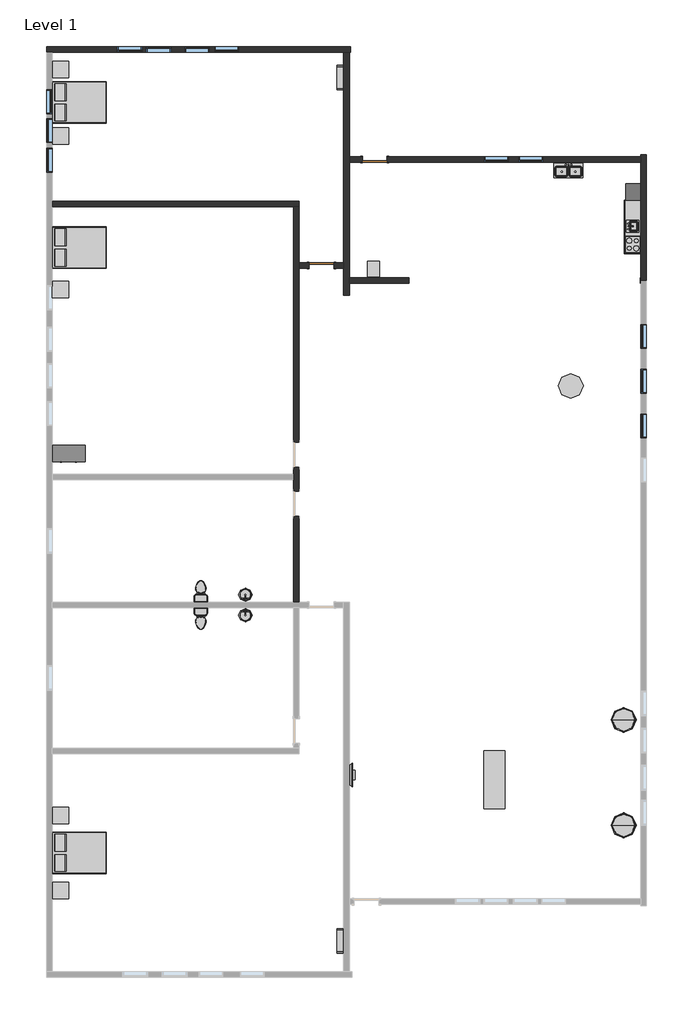
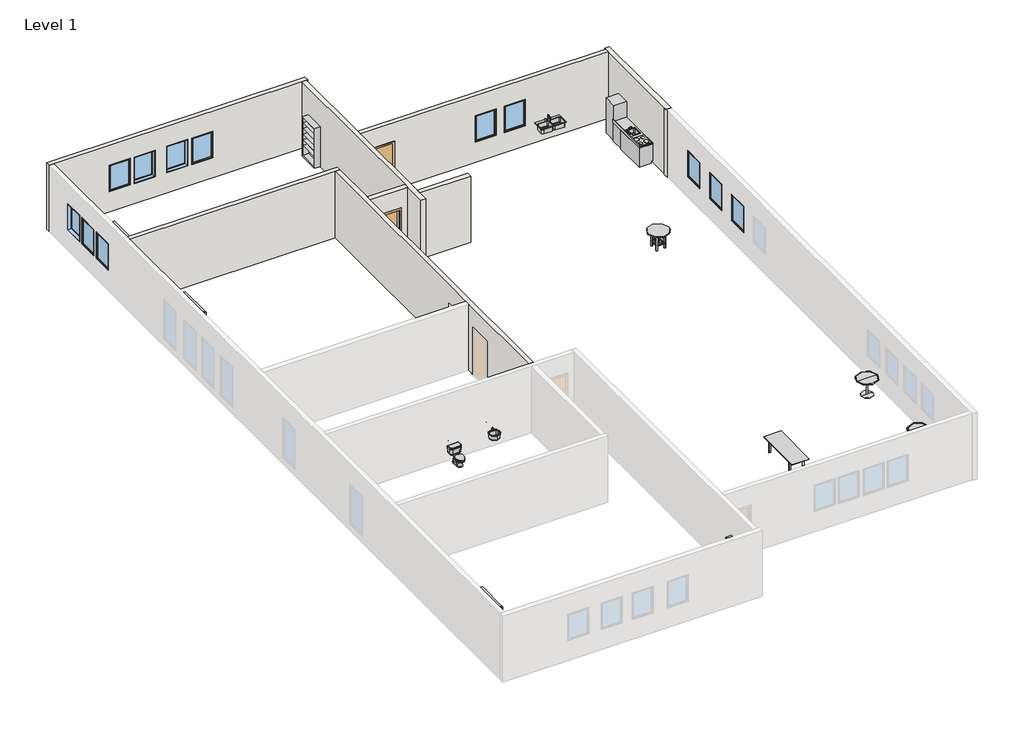
# One storey, part 2 of 2: 17 furniture elements, 12 windows, 9 walls, 6 flow terminals, 5 proxies, 2 doors.
"""IFC4 building model written with IfcOpenShell, lengths in millimetres."""

from ifc_helpers import new_model, si_unit, frame, origin, origin_with_axes, place, context, project, spatial, polyline, outline, extrude, faceted_brep, transform, mapped, element, save
from components import proxy_7e1014cc, proxy_a6faaae8, proxy_45b28599, kitchenette_medium_kitchenette_medium_844211aa, proxy_c523a7b7, door_54dd4da4, flow_terminal_a53be723, flow_terminal_871c2e40, flow_terminal_d49f872f, toilet_domestic_3d_toilet_domestic_3d_f7549cf7, toilet_domestic_3d_toilet_domestic_3d_183bbd19, furniture_c6510c7c, furniture_9fa109b2, m_bed_box_1525_x_2007mm_queen_e2603687, furniture_417d203a, furniture_56245f3a, furniture_92191dda, furniture_905aceb5, furniture_5bc9ed15, furniture_c80d6d9c, window_e2841890

model = new_model("IFC4")

# Units and contexts
model_context = context("Model", 3, world=origin())
ifc_project = project(units=[si_unit("LENGTHUNIT", "METRE", prefix="MILLI")], contexts=[model_context])

# Site, building, storey
site = spatial("IfcSite", under=ifc_project)
building = spatial("IfcBuilding", under=site)
storey = spatial("IfcBuildingStorey", under=building, Name="Level 1", Elevation=0.0)

# Proxies
placement = place(None, origin())
proxy_shape = proxy_7e1014cc(model_context)
element("IfcBuildingElementProxy", 1, Name="18\" x 24\" x 34 1/2\"", ObjectType="18\" x 24\" x 34 1/2\"", at=placement, inside=storey, context=model_context, shape_type="MappedRepresentation", body=[
    mapped(proxy_shape, transform((-2952.3638298, 5873.9040642, 0.0), x_axis=(1.0, 0.0, 0.0), y_axis=(0.0, 1.0, 0.0), z_axis=(0.0, 0.0, 1.0))),
])
proxy_2_shape = proxy_a6faaae8(model_context)
element("IfcBuildingElementProxy", 2, Name="Cook Top-4 Unit2 : 22\" x 20\"", ObjectType="Cook Top-4 Unit2 : 22\" x 20\"", at=placement, inside=storey, context=model_context, shape_type="MappedRepresentation", body=[
    mapped(proxy_2_shape, transform((6922.8887845, 7067.453629, 0.0), x_axis=(0.0, 1.0000000000000002, 0.0), y_axis=(-1.0000000000000002, 0.0, 0.0), z_axis=(0.0, 0.0, 1.0))),
])
proxy_3_shape = proxy_45b28599(model_context)
element("IfcBuildingElementProxy", 3, Name="Dishwasher : 24\" x 24\" x 34\"", ObjectType="Dishwasher : 24\" x 24\" x 34\"", at=placement, inside=storey, context=model_context, shape_type="MappedRepresentation", body=[
    mapped(proxy_3_shape, transform((7214.7383493, 8018.6361605, 0.0), x_axis=(0.0, 1.0000000000000002, 0.0), y_axis=(-1.0000000000000002, 0.0, 0.0), z_axis=(0.0, 0.0, 1.0))),
])
kitchenette_medium_kitchenette_medium_shape = kitchenette_medium_kitchenette_medium_844211aa(model_context)
element("IfcBuildingElementProxy", 4, Name="Kitchenette - Medium : Kitchenette - Medium", ObjectType="Kitchenette - Medium : Kitchenette - Medium", at=placement, inside=storey, context=model_context, shape_type="MappedRepresentation", body=[
    mapped(kitchenette_medium_kitchenette_medium_shape, transform((6618.0887845, 7391.6159241, 0.0), x_axis=(0.0, 1.0000000000000002, 0.0), y_axis=(-1.0000000000000002, 0.0, 0.0), z_axis=(0.0, 0.0, 1.0))),
])
proxy_4_shape = proxy_c523a7b7(model_context)
element("IfcBuildingElementProxy", 5, Name="Refrigerator : 24\" x 25\" LH", ObjectType="Refrigerator : 24\" x 25\" LH", at=placement, inside=storey, context=model_context, shape_type="MappedRepresentation", body=[
    mapped(proxy_4_shape, transform((6968.537756, 9004.203629, 0.0), x_axis=(0.0, 1.0000000000000002, 0.0), y_axis=(-1.0000000000000002, 0.0, 0.0), z_axis=(0.0, 0.0, 1.0))),
])

# Doors
door_shape = door_54dd4da4(model_context)
element("IfcDoor", 6, ObjectType="Single-Flush : 36\" x 84\"", at=placement, inside=storey, context=model_context, shape_type="MappedRepresentation", body=[
    mapped(door_shape, transform((-2602.1112155, 10204.353629, 0.0), x_axis=(-1.0, 0.0, 0.0), y_axis=(0.0, -1.0, 0.0), z_axis=(0.0, 0.0, 1.0))),
])
element("IfcDoor", 7, ObjectType="Single-Flush : 36\" x 84\"", at=placement, inside=storey, context=model_context, shape_type="MappedRepresentation", body=[
    mapped(door_shape, transform((-4570.6112155, 6292.753629, 0.0), x_axis=(1.0, 0.0, 0.0), y_axis=(0.0, 1.0, 0.0), z_axis=(0.0, 0.0, 1.0))),
])

# Flow terminals
flow_terminal_shape = flow_terminal_a53be723(model_context)
element("IfcFlowTerminal", 8, ObjectType="Sink Kitchen-Double : 42\" x 21\"", at=placement, inside=storey, context=model_context, shape_type="MappedRepresentation", body=[
    mapped(flow_terminal_shape, transform((4532.2995439, 9795.6082279, 0.0), x_axis=(1.0, 0.0, 0.0), y_axis=(0.0, 1.0, 0.0), z_axis=(0.0, 0.0, 1.0))),
])
flow_terminal_2_shape = flow_terminal_871c2e40(model_context)
element("IfcFlowTerminal", 9, ObjectType="Sink Kitchen-Island : 18\" x 18\"", at=placement, inside=storey, context=model_context, shape_type="MappedRepresentation", body=[
    mapped(flow_terminal_2_shape, transform((6925.2341856, 7724.8643885, -14.4), x_axis=(0.0, 1.0000000000000002, 0.0), y_axis=(-1.0000000000000002, 0.0, 0.0), z_axis=(0.0, 0.0, 1.0))),
])
flow_terminal_3_shape = flow_terminal_d49f872f(model_context)
element("IfcFlowTerminal", 10, ObjectType="Sink Vanity-Round : 19\" x 19\"", at=placement, inside=storey, context=model_context, shape_type="MappedRepresentation", body=[
    mapped(flow_terminal_3_shape, transform((-7280.659475, -5763.907704, 0.0), x_axis=(-1.0000000000000004, 0.0, 0.0), y_axis=(0.0, -1.0000000000000004, 0.0), z_axis=(0.0, 0.0, 1.0))),
])
element("IfcFlowTerminal", 11, ObjectType="Sink Vanity-Round : 19\" x 19\"", at=placement, inside=storey, context=model_context, shape_type="MappedRepresentation", body=[
    mapped(flow_terminal_3_shape, transform((-7473.9629561, -6694.7566612, 0.0), x_axis=(1.0000000000000002, 0.0, 0.0), y_axis=(0.0, 1.0000000000000002, 0.0), z_axis=(0.0, 0.0, 1.0))),
])
toilet_domestic_3d_toilet_domestic_3d_shape = toilet_domestic_3d_toilet_domestic_3d_f7549cf7(model_context)
toilet_domestic_3d_toilet_domestic_3d_2_shape = toilet_domestic_3d_toilet_domestic_3d_183bbd19(model_context)
element("IfcFlowTerminal", 12, ObjectType="Toilet-Domestic-3D : Toilet-Domestic-3D", at=placement, inside=storey, context=model_context, shape_type="MappedRepresentation", body=[
    mapped(toilet_domestic_3d_toilet_domestic_3d_shape, transform((-9021.7208723, -5633.1503436, 0.0), x_axis=(-1.0000000000000004, 0.0, 0.0), y_axis=(0.0, -1.0000000000000004, 0.0), z_axis=(0.0, 0.0, 1.0))),
    mapped(toilet_domestic_3d_toilet_domestic_3d_2_shape, transform((-9021.7208723, -5633.1503436, 0.0), x_axis=(-1.0000000000000004, 0.0, 0.0), y_axis=(0.0, -1.0000000000000004, 0.0), z_axis=(0.0, 0.0, 1.0))),
])
element("IfcFlowTerminal", 13, ObjectType="Toilet-Domestic-3D : Toilet-Domestic-3D", at=placement, inside=storey, context=model_context, shape_type="MappedRepresentation", body=[
    mapped(toilet_domestic_3d_toilet_domestic_3d_shape, transform((-9021.7208723, -6825.7423983, 0.0), x_axis=(1.0, 0.0, 0.0), y_axis=(0.0, 1.0, 0.0), z_axis=(0.0, 0.0, 1.0))),
    mapped(toilet_domestic_3d_toilet_domestic_3d_2_shape, transform((-9021.7208723, -6825.7423983, 0.0), x_axis=(1.0, 0.0, 0.0), y_axis=(0.0, 1.0, 0.0), z_axis=(0.0, 0.0, 1.0))),
])

# Furniture
furniture_shape = furniture_c6510c7c(model_context)
element("IfcFurniture", 14, ObjectType="Counter Top w Sink Hole : 24\" Depth", at=placement, inside=storey, context=model_context, shape_type="MappedRepresentation", body=[
    mapped(furniture_shape, transform((6618.0887845, 7925.0159241, -14.4), x_axis=(0.0, 1.0000000000000002, 0.0), y_axis=(-1.0000000000000002, 0.0, 0.0), z_axis=(0.0, 0.0, 1.0))),
])
furniture_2_shape = furniture_9fa109b2(model_context)
element("IfcFurniture", 15, ObjectType="Dresser : 48\" x 72\" x 24\"", at=placement, inside=storey, context=model_context, shape_type="MappedRepresentation", body=[
    mapped(furniture_2_shape, transform((-13635.9179557, -278.2834169, 0.0), x_axis=(1.0, 0.0, 0.0), y_axis=(0.0, 1.0, 0.0), z_axis=(0.0, 0.0, 1.0))),
])
m_bed_box_1525_x_2007mm_queen_shape = m_bed_box_1525_x_2007mm_queen_e2603687(model_context)
element("IfcFurniture", 16, ObjectType="M_Bed-Box : 1525 x 2007mm - Queen", at=placement, inside=storey, context=model_context, shape_type="MappedRepresentation", body=[
    mapped(m_bed_box_1525_x_2007mm_queen_shape, transform((-13745.6407237, 11972.90117, 0.0), x_axis=(0.0, 1.0000000000000002, 0.0), y_axis=(-1.0000000000000002, 0.0, 0.0), z_axis=(0.0, 0.0, 1.0))),
])
element("IfcFurniture", 17, ObjectType="M_Bed-Box : 1525 x 2007mm - Queen", at=placement, inside=storey, context=model_context, shape_type="MappedRepresentation", body=[
    mapped(m_bed_box_1525_x_2007mm_queen_shape, transform((-13745.6407237, 6614.50117, 0.0), x_axis=(0.0, 1.0000000000000002, 0.0), y_axis=(-1.0000000000000002, 0.0, 0.0), z_axis=(0.0, 0.0, 1.0))),
])
element("IfcFurniture", 18, ObjectType="M_Bed-Box : 1525 x 2007mm - Queen", at=placement, inside=storey, context=model_context, shape_type="MappedRepresentation", body=[
    mapped(m_bed_box_1525_x_2007mm_queen_shape, transform((-13745.6407237, -15713.09883, 0.0), x_axis=(0.0, 1.0000000000000002, 0.0), y_axis=(-1.0000000000000002, 0.0, 0.0), z_axis=(0.0, 0.0, 1.0))),
])
furniture_3_shape = furniture_417d203a(model_context)
element("IfcFurniture", 19, ObjectType="Shelving : 36\" x 10\" x 72\"", at=placement, inside=storey, context=model_context, shape_type="MappedRepresentation", body=[
    mapped(furniture_3_shape, transform((-4176.9112155, 13226.953629, 0.0), x_axis=(0.0, 1.0, 0.0), y_axis=(-1.0, 0.0, 0.0), z_axis=(0.0, 0.0, 1.0))),
])
element("IfcFurniture", 20, ObjectType="Shelving : 36\" x 10\" x 72\"", at=placement, inside=storey, context=model_context, shape_type="MappedRepresentation", body=[
    mapped(furniture_3_shape, transform((-4176.9112155, -18624.646371, 0.0), x_axis=(0.0, 1.0, 0.0), y_axis=(-1.0, 0.0, 0.0), z_axis=(0.0, 0.0, 1.0))),
])
furniture_4_shape = furniture_56245f3a(model_context)
element("IfcFurniture", 21, ObjectType="TV - Flat Screen : 32\"", at=placement, inside=storey, context=model_context, shape_type="MappedRepresentation", body=[
    mapped(furniture_4_shape, transform((-3483.3725919, -12499.3018568, 0.0), x_axis=(0.0, 1.0000000000000002, 0.0), y_axis=(-1.0000000000000002, 0.0, 0.0), z_axis=(0.0, 0.0, 1.0))),
])
furniture_5_shape = furniture_92191dda(model_context)
element("IfcFurniture", 22, ObjectType="Table-Dining : 30\" x 84\" x 22\"", at=placement, inside=storey, context=model_context, shape_type="MappedRepresentation", body=[
    mapped(furniture_5_shape, transform((1912.6998623, -12699.3121376, 0.0), x_axis=(0.0, 1.0000000000000002, 0.0), y_axis=(-1.0000000000000002, 0.0, 0.0), z_axis=(0.0, 0.0, 1.0))),
])
furniture_6_shape = furniture_905aceb5(model_context)
element("IfcFurniture", 23, ObjectType="Table-Dining Round w Chairs : 36\" Diameter", at=placement, inside=storey, context=model_context, shape_type="MappedRepresentation", body=[
    mapped(furniture_6_shape, transform((4533.2068173, 2032.6323176, 0.0), x_axis=(1.0, 0.0, 0.0), y_axis=(0.0, 1.0, 0.0), z_axis=(0.0, 0.0, 1.0))),
])
furniture_7_shape = furniture_5bc9ed15(model_context)
element("IfcFurniture", 24, ObjectType="Table-Night Stand : 24\" x 24\" x 30\"", at=placement, inside=storey, context=model_context, shape_type="MappedRepresentation", body=[
    mapped(furniture_7_shape, transform((-14518.4448458, 10763.153629, 0.0), x_axis=(1.0, 0.0, 0.0), y_axis=(0.0, 1.0, 0.0), z_axis=(0.0, 0.0, 1.0))),
])
element("IfcFurniture", 25, ObjectType="Table-Night Stand : 24\" x 24\" x 30\"", at=placement, inside=storey, context=model_context, shape_type="MappedRepresentation", body=[
    mapped(furniture_7_shape, transform((-14518.4448458, 13226.953629, 0.0), x_axis=(1.0, 0.0, 0.0), y_axis=(0.0, 1.0, 0.0), z_axis=(0.0, 0.0, 1.0))),
])
element("IfcFurniture", 26, ObjectType="Table-Night Stand : 24\" x 24\" x 30\"", at=placement, inside=storey, context=model_context, shape_type="MappedRepresentation", body=[
    mapped(furniture_7_shape, transform((-14518.4448458, 5098.953629, 0.0), x_axis=(1.0, 0.0, 0.0), y_axis=(0.0, 1.0, 0.0), z_axis=(0.0, 0.0, 1.0))),
])
element("IfcFurniture", 27, ObjectType="Table-Night Stand : 24\" x 24\" x 30\"", at=placement, inside=storey, context=model_context, shape_type="MappedRepresentation", body=[
    mapped(furniture_7_shape, transform((-14518.4448458, -14306.646371, 0.0), x_axis=(1.0, 0.0, 0.0), y_axis=(0.0, 1.0, 0.0), z_axis=(0.0, 0.0, 1.0))),
])
element("IfcFurniture", 28, ObjectType="Table-Night Stand : 24\" x 24\" x 30\"", at=placement, inside=storey, context=model_context, shape_type="MappedRepresentation", body=[
    mapped(furniture_7_shape, transform((-14518.4448458, -17075.246371, 0.0), x_axis=(1.0, 0.0, 0.0), y_axis=(0.0, 1.0, 0.0), z_axis=(0.0, 0.0, 1.0))),
])
furniture_8_shape = furniture_c80d6d9c(model_context)
element("IfcFurniture", 29, ObjectType="Table-Round : 36\" Diameter", at=placement, inside=storey, context=model_context, shape_type="MappedRepresentation", body=[
    mapped(furniture_8_shape, transform((6592.6887845, -14357.446371, 0.0), x_axis=(1.0, 0.0, 0.0), y_axis=(0.0, 1.0, 0.0), z_axis=(0.0, 0.0, 1.0))),
])
element("IfcFurniture", 30, ObjectType="Table-Round : 36\" Diameter", at=placement, inside=storey, context=model_context, shape_type="MappedRepresentation", body=[
    mapped(furniture_8_shape, transform((6592.6887845, -10471.246371, 0.0), x_axis=(1.0, 0.0, 0.0), y_axis=(0.0, 1.0, 0.0), z_axis=(0.0, 0.0, 1.0))),
])

# Walls
element("IfcWall", 31, ObjectType="Generic - 8\"", at=placement, inside=storey, context=model_context, shape_type="Brep", body=[
    faceted_brep([(-14717.9112155, 14166.753629, 0.0), (-14514.7112155, 14166.753629, 0.0), (-3745.1112155, 14166.753629, 0.0), (-3541.9112155, 14166.753629, 0.0), (-3491.1112155, 14166.753629, 0.0), (-3491.1112155, 14166.753629, 3048.0), (-3541.9112155, 14166.753629, 3048.0), (-3745.1112155, 14166.753629, 3048.0), (-14514.7112155, 14166.753629, 3048.0), (-14717.9112155, 14166.753629, 3048.0), (-12101.7112155, 14166.753629, 2133.6), (-11187.3112155, 14166.753629, 2133.6), (-11187.3112155, 14166.753629, 914.4), (-12101.7112155, 14166.753629, 914.4), (-10120.5112155, 14166.753629, 2133.6), (-10120.5112155, 14166.753629, 914.4), (-11034.9112155, 14166.753629, 914.4), (-11034.9112155, 14166.753629, 2133.6), (-8698.1112155, 14166.753629, 2133.6), (-8698.1112155, 14166.753629, 914.4), (-9612.5112155, 14166.753629, 914.4), (-9612.5112155, 14166.753629, 2133.6), (-8520.3112155, 14166.753629, 2133.6), (-7605.9112155, 14166.753629, 2133.6), (-7605.9112155, 14166.753629, 914.4), (-8520.3112155, 14166.753629, 914.4), (-14717.9112155, 14369.953629, 0.0), (-14717.9112155, 14369.953629, 3048.0), (-3491.1112155, 14369.953629, 3048.0), (-3491.1112155, 14369.953629, 0.0), (-12101.7112155, 14369.953629, 2133.6), (-12101.7112155, 14369.953629, 914.4), (-11187.3112155, 14369.953629, 914.4), (-11187.3112155, 14369.953629, 2133.6), (-10120.5112155, 14369.953629, 2133.6), (-11034.9112155, 14369.953629, 2133.6), (-11034.9112155, 14369.953629, 914.4), (-10120.5112155, 14369.953629, 914.4), (-8698.1112155, 14369.953629, 2133.6), (-9612.5112155, 14369.953629, 2133.6), (-9612.5112155, 14369.953629, 914.4), (-8698.1112155, 14369.953629, 914.4), (-8520.3112155, 14369.953629, 2133.6), (-8520.3112155, 14369.953629, 914.4), (-7605.9112155, 14369.953629, 914.4), (-7605.9112155, 14369.953629, 2133.6)], [[[0, 1, 2, 3, 4, 5, 6, 7, 8, 9], [10, 11, 12, 13], [14, 15, 16, 17], [18, 19, 20, 21], [22, 23, 24, 25]], [[26, 27, 28, 29], [30, 31, 32, 33], [34, 35, 36, 37], [38, 39, 40, 41], [42, 43, 44, 45]], [[4, 3, 2, 1, 0, 26, 29]], [[5, 4, 29, 28]], [[9, 8, 7, 6, 5, 28, 27]], [[0, 9, 27, 26]], [[31, 30, 10, 13]], [[32, 31, 13, 12]], [[33, 32, 12, 11]], [[30, 33, 11, 10]], [[15, 14, 34, 37]], [[16, 15, 37, 36]], [[17, 16, 36, 35]], [[14, 17, 35, 34]], [[19, 18, 38, 41]], [[20, 19, 41, 40]], [[21, 20, 40, 39]], [[18, 21, 39, 38]], [[43, 42, 22, 25]], [[44, 43, 25, 24]], [[45, 44, 24, 23]], [[42, 45, 23, 22]]]),
])
element("IfcWall", 32, ObjectType="Generic - 8\"", at=placement, inside=storey, context=model_context, shape_type="Brep", body=[
    faceted_brep([(-3745.1112155, 14166.753629, 0.0), (-3745.1112155, 6394.353629, 0.0), (-3745.1112155, 6191.153629, 0.0), (-3745.1112155, 5200.553629, 0.0), (-3745.1112155, 5200.553629, 3048.0), (-3745.1112155, 6191.153629, 3048.0), (-3745.1112155, 6394.353629, 3048.0), (-3745.1112155, 14166.753629, 3048.0), (-3541.9112155, 14166.753629, 0.0), (-3541.9112155, 14166.753629, 3048.0), (-3541.9112155, 10305.953629, 3048.0), (-3541.9112155, 10102.753629, 3048.0), (-3541.9112155, 5835.553629, 3048.0), (-3541.9112155, 5632.353629, 3048.0), (-3541.9112155, 5200.553629, 3048.0), (-3541.9112155, 5200.553629, 0.0), (-3541.9112155, 5632.353629, 0.0), (-3541.9112155, 5835.553629, 0.0), (-3541.9112155, 10102.753629, 0.0), (-3541.9112155, 10305.953629, 0.0)], [[[0, 1, 2, 3, 4, 5, 6, 7]], [[8, 9, 10, 11, 12, 13, 14, 15, 16, 17, 18, 19]], [[3, 2, 1, 0, 8, 19, 18, 17, 16, 15]], [[4, 3, 15, 14]], [[7, 6, 5, 4, 14, 13, 12, 11, 10, 9]], [[0, 7, 9, 8]]]),
])
element("IfcWall", 33, ObjectType="Generic - 8\"", at=placement, inside=storey, context=model_context, shape_type="SweptSolid", body=[
    extrude(outline(polyline([(0.0, -3541.9112155), (0.0, -3059.3112155), (2133.6, -3059.3112155), (2133.6, -2144.9112155), (0.0, -2144.9112155), (0.0, 7227.6887845), (3048.0, 7227.6887845), (3048.0, -3541.9112155), (0.0, -3541.9112155)]), holes=[polyline([(2133.6, 1436.4887845), (2133.6, 2350.8887845), (914.4, 2350.8887845), (914.4, 1436.4887845), (2133.6, 1436.4887845)]), polyline([(2133.6, 2706.4887845), (2133.6, 3620.8887845), (914.4, 3620.8887845), (914.4, 2706.4887845), (2133.6, 2706.4887845)])]), frame((0.0, 10102.753629, 0.0), z_axis=(0.0, 1.0, 0.0), x_axis=(0.0, 0.0, 1.0)), (0.0, 0.0, 1.0), 203.2),
])
element("IfcWall", 34, ObjectType="Generic - 8\"", at=placement, inside=storey, context=model_context, shape_type="SweptSolid", body=[
    extrude(outline(polyline([(-1332.1112155, 5632.353629), (-3541.9112155, 5632.353629), (-3541.9112155, 5835.553629), (-1332.1112155, 5835.553629), (-1332.1112155, 5632.353629)])), origin_with_axes(), (0.0, 0.0, 1.0), 3048.0),
])
element("IfcWall", 35, ObjectType="Generic - 8\"", at=placement, inside=storey, context=model_context, shape_type="Brep", body=[
    faceted_brep([(-14514.7112155, 8451.753629, 0.0), (-5599.3112155, 8451.753629, 0.0), (-5396.1112155, 8451.753629, 0.0), (-5396.1112155, 8451.753629, 3048.0), (-5599.3112155, 8451.753629, 3048.0), (-14514.7112155, 8451.753629, 3048.0), (-14514.7112155, 8654.953629, 0.0), (-14514.7112155, 8654.953629, 3048.0), (-5396.1112155, 8654.953629, 3048.0), (-5396.1112155, 8654.953629, 0.0)], [[[0, 1, 2, 3, 4, 5]], [[6, 7, 8, 9]], [[2, 1, 0, 6, 9]], [[5, 4, 3, 8, 7]], [[0, 5, 7, 6]], [[3, 2, 9, 8]]]),
])
element("IfcWall", 36, ObjectType="Generic - 8\"", at=placement, inside=storey, context=model_context, shape_type="Brep", body=[
    faceted_brep([(-5599.3112155, -1149.446371, 2133.6), (-5599.3112155, -1149.446371, 0.0), (-5599.3112155, -1403.446371, 0.0), (-5599.3112155, -1606.646371, 0.0), (-5599.3112155, -2038.446371, 0.0), (-5599.3112155, -2038.446371, 2133.6), (-5599.3112155, -2952.846371, 2133.6), (-5599.3112155, -2952.846371, 0.0), (-5599.3112155, -6127.846371, 0.0), (-5599.3112155, -6127.846371, 3048.0), (-5599.3112155, -1606.646371, 3048.0), (-5599.3112155, -1403.446371, 3048.0), (-5599.3112155, 8451.753629, 3048.0), (-5599.3112155, 8451.753629, 0.0), (-5599.3112155, -235.046371, 0.0), (-5599.3112155, -235.046371, 2133.6), (-5396.1112155, -2038.446371, 0.0), (-5396.1112155, -1149.446371, 0.0), (-5396.1112155, -1149.446371, 2133.6), (-5396.1112155, -235.046371, 2133.6), (-5396.1112155, -235.046371, 0.0), (-5396.1112155, 6191.153629, 0.0), (-5396.1112155, 6394.353629, 0.0), (-5396.1112155, 8451.753629, 0.0), (-5396.1112155, 8451.753629, 3048.0), (-5396.1112155, 6394.353629, 3048.0), (-5396.1112155, 6191.153629, 3048.0), (-5396.1112155, -6127.846371, 3048.0), (-5396.1112155, -6127.846371, 0.0), (-5396.1112155, -2952.846371, 0.0), (-5396.1112155, -2952.846371, 2133.6), (-5396.1112155, -2038.446371, 2133.6)], [[[0, 1, 2, 3, 4, 5, 6, 7, 8, 9, 10, 11, 12, 13, 14, 15]], [[16, 17, 18, 19, 20, 21, 22, 23, 24, 25, 26, 27, 28, 29, 30, 31]], [[29, 28, 8, 7]], [[14, 13, 23, 22, 21, 20]], [[4, 3, 2, 1, 17, 16]], [[12, 11, 10, 9, 27, 26, 25, 24]], [[13, 12, 24, 23]], [[9, 8, 28, 27]], [[5, 4, 16, 31]], [[6, 5, 31, 30]], [[7, 6, 30, 29]], [[18, 17, 1, 0]], [[19, 18, 0, 15]], [[20, 19, 15, 14]]]),
])
element("IfcWall", 37, ObjectType="Generic - 8\"", at=placement, inside=storey, context=model_context, shape_type="SweptSolid", body=[
    extrude(outline(polyline([(2133.6, -4113.4112155), (0.0, -4113.4112155), (0.0, -3745.1112155), (3048.0, -3745.1112155), (3048.0, -5396.1112155), (0.0, -5396.1112155), (0.0, -5027.8112155), (2133.6, -5027.8112155), (2133.6, -4113.4112155)])), frame((0.0, 6191.153629, 0.0), z_axis=(0.0, 1.0, 0.0), x_axis=(0.0, 0.0, 1.0)), (0.0, 0.0, 1.0), 203.2),
])
element("IfcWall", 38, ObjectType="Generic - 8\"", at=placement, inside=storey, context=model_context, shape_type="Brep", body=[
    faceted_brep([(7202.2887845, 5632.353629, 0.0), (7227.6887845, 5632.353629, 0.0), (7227.6887845, 5632.353629, 3048.0), (7202.2887845, 5632.353629, 3048.0), (7202.2887845, 5835.553629, 0.0), (7202.2887845, 5835.553629, 3048.0), (7227.6887845, 5835.553629, 3048.0), (7227.6887845, 5835.553629, 0.0), (7227.6887845, 5733.953629, 0.0), (7227.6887845, 5733.953629, 3048.0)], [[[0, 1, 2, 3]], [[4, 5, 6, 7]], [[1, 0, 4, 7, 8]], [[3, 2, 9, 6, 5]], [[0, 3, 5, 4]], [[2, 1, 8, 7, 6, 9]]]),
])
element("IfcWall", 39, ObjectType="Generic - 8\"", at=placement, inside=storey, context=model_context, shape_type="Brep", body=[
    faceted_brep([(7227.6887845, 10382.153629, 0.0), (7227.6887845, 10305.953629, 0.0), (7227.6887845, 10102.753629, 0.0), (7227.6887845, 5835.553629, 0.0), (7227.6887845, 5733.953629, 0.0), (7227.6887845, 5733.953629, 3048.0), (7227.6887845, 5835.553629, 3048.0), (7227.6887845, 10102.753629, 3048.0), (7227.6887845, 10305.953629, 3048.0), (7227.6887845, 10382.153629, 3048.0), (7430.8887845, 10382.153629, 0.0), (7430.8887845, 10382.153629, 3048.0), (7430.8887845, 5733.953629, 3048.0), (7430.8887845, 5733.953629, 0.0)], [[[0, 1, 2, 3, 4, 5, 6, 7, 8, 9]], [[10, 11, 12, 13]], [[4, 3, 2, 1, 0, 10, 13]], [[5, 4, 13, 12]], [[9, 8, 7, 6, 5, 12, 11]], [[0, 9, 11, 10]]]),
])

# Windows
window_shape = window_e2841890(model_context)
element("IfcWindow", 40, ObjectType="Fixed : 36\" x 48\"", at=placement, inside=storey, context=model_context, shape_type="MappedRepresentation", body=[
    mapped(window_shape, transform((-14616.3112155, 12299.853629, 0.0), x_axis=(0.0, -1.0, 0.0), y_axis=(1.0, 0.0, 0.0), z_axis=(0.0, 0.0, 1.0))),
])
element("IfcWindow", 41, ObjectType="Fixed : 36\" x 48\"", at=placement, inside=storey, context=model_context, shape_type="MappedRepresentation", body=[
    mapped(window_shape, transform((-14616.3112155, 11309.253629, 0.0), x_axis=(0.0, 1.0, 0.0), y_axis=(-1.0, 0.0, 0.0), z_axis=(0.0, 0.0, 1.0))),
])
element("IfcWindow", 42, ObjectType="Fixed : 36\" x 48\"", at=placement, inside=storey, context=model_context, shape_type="MappedRepresentation", body=[
    mapped(window_shape, transform((-14616.3112155, 10217.053629, 0.0), x_axis=(0.0, 1.0, 0.0), y_axis=(-1.0, 0.0, 0.0), z_axis=(0.0, 0.0, 1.0))),
])
element("IfcWindow", 43, ObjectType="Fixed : 36\" x 48\"", at=placement, inside=storey, context=model_context, shape_type="MappedRepresentation", body=[
    mapped(window_shape, transform((-11682.6112155, 14268.353629, 0.0), x_axis=(-1.0, 0.0, 0.0), y_axis=(0.0, -1.0, 0.0), z_axis=(0.0, 0.0, 1.0))),
])
element("IfcWindow", 44, ObjectType="Fixed : 36\" x 48\"", at=placement, inside=storey, context=model_context, shape_type="MappedRepresentation", body=[
    mapped(window_shape, transform((-10539.6112155, 14268.353629, 0.0), x_axis=(1.0, 0.0, 0.0), y_axis=(0.0, 1.0, 0.0), z_axis=(0.0, 0.0, 1.0))),
])
element("IfcWindow", 45, ObjectType="Fixed : 36\" x 48\"", at=placement, inside=storey, context=model_context, shape_type="MappedRepresentation", body=[
    mapped(window_shape, transform((-9117.2112155, 14268.353629, 0.0), x_axis=(1.0, 0.0, 0.0), y_axis=(0.0, 1.0, 0.0), z_axis=(0.0, 0.0, 1.0))),
])
element("IfcWindow", 46, ObjectType="Fixed : 36\" x 48\"", at=placement, inside=storey, context=model_context, shape_type="MappedRepresentation", body=[
    mapped(window_shape, transform((-8101.2112155, 14268.353629, 0.0), x_axis=(-1.0, 0.0, 0.0), y_axis=(0.0, -1.0, 0.0), z_axis=(0.0, 0.0, 1.0))),
])
element("IfcWindow", 47, ObjectType="Fixed : 36\" x 48\"", at=placement, inside=storey, context=model_context, shape_type="MappedRepresentation", body=[
    mapped(window_shape, transform((1855.5887845, 10204.353629, 0.0), x_axis=(-1.0, 0.0, 0.0), y_axis=(0.0, -1.0, 0.0), z_axis=(0.0, 0.0, 1.0))),
])
element("IfcWindow", 48, ObjectType="Fixed : 36\" x 48\"", at=placement, inside=storey, context=model_context, shape_type="MappedRepresentation", body=[
    mapped(window_shape, transform((3125.5887845, 10204.353629, 0.0), x_axis=(-1.0, 0.0, 0.0), y_axis=(0.0, -1.0, 0.0), z_axis=(0.0, 0.0, 1.0))),
])
element("IfcWindow", 49, ObjectType="Fixed : 36\" x 48\"", at=placement, inside=storey, context=model_context, shape_type="MappedRepresentation", body=[
    mapped(window_shape, transform((7329.2887845, 3714.653629, 0.0), x_axis=(0.0, 1.0, 0.0), y_axis=(-1.0, 0.0, 0.0), z_axis=(0.0, 0.0, 1.0))),
])
element("IfcWindow", 50, ObjectType="Fixed : 36\" x 48\"", at=placement, inside=storey, context=model_context, shape_type="MappedRepresentation", body=[
    mapped(window_shape, transform((7329.2887845, 2063.653629, 0.0), x_axis=(0.0, 1.0, 0.0), y_axis=(-1.0, 0.0, 0.0), z_axis=(0.0, 0.0, 1.0))),
])
element("IfcWindow", 51, ObjectType="Fixed : 36\" x 48\"", at=placement, inside=storey, context=model_context, shape_type="MappedRepresentation", body=[
    mapped(window_shape, transform((7329.2887845, 412.653629, 0.0), x_axis=(0.0, 1.0, 0.0), y_axis=(-1.0, 0.0, 0.0), z_axis=(0.0, 0.0, 1.0))),
])

save(model, "model.ifc")

# Revit data of these elements
# Type "18\" x 24\" x 34 1/2\""
#   Label = "T"
#   Assembly Code = "E1090400"
#   Depth = 2' - 0"
#   Height = 2' - 10 1/2"
#   Width = 1' - 6"
#   Panel Face Material = Plastic, Opaque Black
#   Trach Compact. Material = Steel, Paint Finish, Ivory, Matte
#   Default Elevation = 0
# Type "Cook Top-4 Unit2 : 22\" x 20\""
#   Depth = 1' - 8"
#   Width = 1' - 10"
#   Burner Material = Steel, Chrome Plated
#   Cooktop Material = Steel, Polished
#   Default Elevation = 0
#   Assembly Code = ""
# Type "Dishwasher : 24\" x 24\" x 34\""
#   Label = "DW"
#   Assembly Code = "E1090400"
#   Depth = 2' - 0"
#   Height = 2' - 10"
#   Width = 2' - 0"
#   Dishwasher Material = Steel, Paint Finish, Ivory, Glossy
#   Panel Face Material = Plastic, Opaque Black
#   Default Elevation = 0
# Type "Kitchenette - Medium : Kitchenette - Medium"
#   Assembly Code = "E1090400"
#   Counter Length = 6' - 6"
#   Cabinet Width = 4' - 6"
#   Cabinet Height = 2' - 10 1/2"
#   Cabinet Depth = 2' - 0"
#   Toe Depth = 0' - 3"
#   Toe Height = 0' - 3 1/2"
#   Cabinet Material = Cabinets
#   Door/Drawer Material = Cabinets
#   Handle Material = Cabinets - Handles
#   Default Elevation = 0
# Type "Refrigerator : 24\" x 25\" LH"
#   Label = "REF."
#   Assembly Code = "E1090400"
#   Depth = 2' - 0 3/4"
#   Handle = 0' - 1 1/2"
#   Height = 5' - 3 1/2"
#   Rear Clearance = 0' - 2"
#   Top Door Height = 1' - 8"
#   Width = 1' - 11 1/2"
#   Material = Steel, Paint Finish, Ivory, Glossy
#   Default Elevation = 0
# Type "Single-Flush : 36\" x 84\""
#   Type Mark = "1"
#   Construction Type Id = "MDOOR"
#   Assembly Code = "C1020"
#   Analytic Construction = "Metal"
#   Thickness = 0' - 2"
#   Heat Transfer Coefficient (U) = 0.651978 BTU/(h·ft²·°F)
#   Height = 7' - 0"
#   Trim Projection Ext = 0' - 1"
#   Trim Projection Int = 0' - 1"
#   Trim Width = 0' - 3"
#   Width = 3' - 0"
#   Define Thermal Properties by = 1
#   Door Material = Door - Panel
#   Frame Material = Door - Frame
#   Visual Light Transmittance = 0
#   Solar Heat Gain Coefficient = 0
#   Function = (empty or 0)
#   Wall Closure = (empty or 0)
# Type "Sink Kitchen-Double : 42\" x 21\""
#   Assembly Code = "D2010410"
#   Counter Height = 3' - 0"
#   Depth = 1' - 9"
#   Width = 3' - 6"
#   Faucet Material = Steel, Polished
#   Sink Material = Steel, Polished
#   Default Elevation = 0
# Type "Sink Kitchen-Island : 18\" x 18\""
#   Assembly Code = "D2010410"
#   Counter Height = 3' - 0"
#   Depth = 1' - 6"
#   Width = 1' - 6"
#   Faucet Material = Steel, Polished
#   Sink Material = Steel, Polished
#   Default Elevation = 0
# Type "Sink Vanity-Round : 19\" x 19\""
#   Assembly Code = "D2010400"
#   Top Of Counter = 2' - 7"
#   Basin Material = Porcelain, Linen
#   Faucet Material = Steel, Polished
#   Default Elevation = 0
# Type "Toilet-Domestic-3D : Toilet-Domestic-3D"
#   Assembly Code = "D2010110"
#   Toilet - Bowl/Basin Material = Porcelain, Linen
#   Toilet - Seat Material = Laminate, Linen, Matte
#   Default Elevation = 0
# Type "Counter Top w Sink Hole : 24\" Depth"
#   Assembly Code = "C1030400"
#   Counter Thickness = 0' - 1 1/2"
#   Depth = 2' - 1"
#   Height = 3' - 0"
#   Length [instance default] = 8' - 0"
#   Sink Location [instance default] = 2' - 0"
#   Sink Location To Wall [instance default] = 0' - 6"
#   Sink Opening Depth [instance default] = 1' - 3"
#   Sink Opening Width [instance default] = 2' - 3"
#   Counter Top Material = none
#   Default Elevation = 0
# Type "Dresser : 48\" x 72\" x 24\""
#   Assembly Code = "E2020200"
#   Depth = 2' - 0"
#   Height = 6' - 0"
#   Width = 4' - 0"
#   Dresser Material = Laminate - Ivory, Glossy
#   Drawer Material = Laminate, Ivory, Matte
#   Knob Material = Cherry
#   Default Elevation = 0
# Type "M_Bed-Box : 1525 x 2007mm - Queen"
#   Length = 6' - 7.01575"
#   Width = 5' - 0.03937"
#   Frame Material = Birch
#   Mattress Material = Linen, White
#   Default Elevation = 0
# Type "Shelving : 36\" x 10\" x 72\""
#   Assembly Code = "E2020200"
#   Depth = 0' - 10"
#   Height = 6' - 0"
#   Width = 3' - 0"
#   Shelving Unit Material = Birch
#   Default Elevation = 0
# Type "TV - Flat Screen : 32\""
#   SinAng = 0' - 0.0193"
#   L = 2' - 3.79372"
#   H = 1' - 3.6354"
#   Thickness = 0' - 4.33071"
#   Diagonal = 2' - 7.88976"
#   CosAng = 0' - 0.03431"
#   Stand [instance default] = yes
#   Default Elevation = 0
# Type "Table-Dining : 30\" x 84\" x 22\""
#   Assembly Code = "E2020200"
#   Height = 1' - 10"
#   Length = 7' - 0"
#   Width = 2' - 6"
#   Base Material = Steel, Chrome Plated
#   Top Material = Glass - Clear, Grey
#   Default Elevation = 0
# Type "Table-Dining Round w Chairs : 36\" Diameter"
#   Assembly Code = "E2020200"
#   Radius = 1' - 6"
#   Diameter = 3' - 0"
#   Height = 2' - 6"
#   Chairs = 4
#   Base Material = Pine
#   Top Material = Laminate, Linen, Matte
#   Default Elevation = 0
# Type "Table-Night Stand : 24\" x 24\" x 30\""
#   Assembly Code = "E2020200"
#   Depth = 2' - 0"
#   Height = 2' - 6"
#   Width = 2' - 0"
#   Base Material = Birch
#   Top Material = Laminate, Ivory, Matte
#   Default Elevation = 0
# Type "Table-Round : 36\" Diameter"
#   Assembly Code = "E2020200"
#   Base Radius = 0' - 10"
#   Height = 2' - 6"
#   Radius = 1' - 6"
#   Base Material = Steel, Chrome Plated
#   Top Material = Birch
#   Default Elevation = 0
# Type "Generic - 8\""
#   Assembly Code = "B2010"
#   Layers, outside or top first: 0' - 8" no material (function 1)
# Type "Fixed : 36\" x 48\""
#   Type Mark = "1"
#   Construction Type Id = "GSP4R"
#   Assembly Code = "B2020100"
#   Analytic Construction = "1/8 in Pilkington single glazing"
#   Visual Light Transmittance = 0.9
#   Solar Heat Gain Coefficient = 0.78
#   Heat Transfer Coefficient (U) = 0.6496 BTU/(h·ft²·°F)
#   Height = 4' - 0"
#   Default Sill Height = 3' - 0"
#   Width = 3' - 0"
#   Window Inset = 0' - 0 3/4"
#   Define Thermal Properties by = 1
#   Glass Pane Material = Glass
#   Sash Material = Sash
#   Wall Closure = (empty or 0)
# Element 1 (IfcBuildingElementProxy, "18\" x 24\" x 34 1/2\"")
#   Phase Created = New Construction
#   Materials on its faces: "Steel, Paint Finish, Ivory, Matte", "Plastic, Opaque Black"
# Element 2 (IfcBuildingElementProxy, "Cook Top-4 Unit2 : 22\" x 20\"")
#   Phase Created = New Construction
#   Materials on its faces: "Steel, Chrome Plated", "Steel, Polished"
# Element 3 (IfcBuildingElementProxy, "Dishwasher : 24\" x 24\" x 34\"")
#   Phase Created = New Construction
#   Materials on its faces: "Steel, Paint Finish, Ivory, Glossy", "Plastic, Opaque Black"
# Element 4 (IfcBuildingElementProxy, "Kitchenette - Medium : Kitchenette - Medium")
#   Phase Created = New Construction
#   Materials on its faces: "Cabinets", "Cabinets - Handles"
# Element 5 (IfcBuildingElementProxy, "Refrigerator : 24\" x 25\" LH")
#   Phase Created = New Construction
#   Materials on its faces: "Steel, Paint Finish, Ivory, Glossy", "Steel, Chrome Plated"
# Elements 6, 7 (IfcDoor, "Single-Flush : 36\" x 84\"")
#   Phase Created = New Construction
#   Materials on its faces: "Door - Frame", "Door - Panel"
# Element 8 (IfcFlowTerminal, "Sink Kitchen-Double : 42\" x 21\"")
#   Mark = "8"
#   Phase Created = New Construction
#   Materials on its faces: "Steel, Polished"
# Element 9 (IfcFlowTerminal, "Sink Kitchen-Island : 18\" x 18\"")
#   Mark = "7"
#   Phase Created = New Construction
#   Materials on its faces: "Steel, Polished"
# Element 10 (IfcFlowTerminal, "Sink Vanity-Round : 19\" x 19\"")
#   Mark = "5"
#   Phase Created = New Construction
#   Materials on its faces: "Porcelain, Linen", "Steel, Polished"
# Element 11 (IfcFlowTerminal, "Sink Vanity-Round : 19\" x 19\"")
#   Mark = "6"
#   Phase Created = New Construction
#   Materials on its faces: "Porcelain, Linen", "Steel, Polished"
# Element 12 (IfcFlowTerminal, "Toilet-Domestic-3D : Toilet-Domestic-3D")
#   Mark = "3"
#   Phase Created = New Construction
#   Materials on its faces: "Porcelain, Linen", "Laminate, Linen, Matte"
# Element 13 (IfcFlowTerminal, "Toilet-Domestic-3D : Toilet-Domestic-3D")
#   Mark = "4"
#   Phase Created = New Construction
#   Materials on its faces: "Porcelain, Linen", "Laminate, Linen, Matte"
# Element 14 (IfcFurniture, "Counter Top w Sink Hole : 24\" Depth")
#   Sink Opening Depth = 1' - 2"
#   Sink Location To Wall = 0' - 6"
#   Length = 6' - 6"
#   Sink Location = 3' - 4"
#   Sink Opening Width = 1' - 4"
#   Phase Created = New Construction
#   Materials on its faces: "Counter Top"
# Element 15 (IfcFurniture, "Dresser : 48\" x 72\" x 24\"")
#   Phase Created = New Construction
#   Materials on its faces: "Laminate, Ivory, Matte", "Cherry", "Laminate - Ivory, Glossy"
# Elements 16, 17, 18 (IfcFurniture, "M_Bed-Box : 1525 x 2007mm - Queen")
#   Phase Created = New Construction
#   Materials on its faces: "Birch", "Linen, White"
# Elements 19, 20 (IfcFurniture, "Shelving : 36\" x 10\" x 72\"")
#   Phase Created = New Construction
#   Materials on its faces: "Birch"
# Element 21 (IfcFurniture, "TV - Flat Screen : 32\"")
#   Stand = yes
#   Phase Created = New Construction
#   Materials on its faces: "TV - Black", "TV - Glass", "TV - Screen"
# Element 22 (IfcFurniture, "Table-Dining : 30\" x 84\" x 22\"")
#   Phase Created = New Construction
#   Materials on its faces: "Steel, Chrome Plated", "Glass - Clear, Grey"
# Element 23 (IfcFurniture, "Table-Dining Round w Chairs : 36\" Diameter")
#   Phase Created = New Construction
#   Materials on its faces: "Pine", "Laminate, Linen, Matte"
# Elements 24, 25, 26, 27, 28 (IfcFurniture, "Table-Night Stand : 24\" x 24\" x 30\"")
#   Phase Created = New Construction
#   Materials on its faces: "Birch", "Laminate, Ivory, Matte"
# Elements 29, 30 (IfcFurniture, "Table-Round : 36\" Diameter")
#   Phase Created = New Construction
#   Materials on its faces: "Steel, Chrome Plated", "Birch"
# Elements 31, 32, 33, 34, 35, 36, 37, 38, 39 (IfcWall, "Generic - 8\"")
#   Top Offset = 0' - 0"
#   Base Offset = 0' - 0"
#   Unconnected Height = 10' - 0"
#   wall height = 10' - 0"
#   Phase Created = New Construction
#   Base Constraint = Level 1
#   Materials on its faces: "Default Wall"
# Element 40 (IfcWindow, "Fixed : 36\" x 48\"")
#   Mark = "1"
#   Phase Created = New Construction
#   Materials on its faces: "Sash", "Glass"
# Element 41 (IfcWindow, "Fixed : 36\" x 48\"")
#   Mark = "2"
#   Phase Created = New Construction
#   Materials on its faces: "Sash", "Glass"
# Element 42 (IfcWindow, "Fixed : 36\" x 48\"")
#   Mark = "3"
#   Phase Created = New Construction
#   Materials on its faces: "Sash", "Glass"
# Element 43 (IfcWindow, "Fixed : 36\" x 48\"")
#   Mark = "4"
#   Phase Created = New Construction
#   Materials on its faces: "Sash", "Glass"
# Element 44 (IfcWindow, "Fixed : 36\" x 48\"")
#   Mark = "5"
#   Phase Created = New Construction
#   Materials on its faces: "Sash", "Glass"
# Element 45 (IfcWindow, "Fixed : 36\" x 48\"")
#   Mark = "6"
#   Phase Created = New Construction
#   Materials on its faces: "Sash", "Glass"
# Element 46 (IfcWindow, "Fixed : 36\" x 48\"")
#   Mark = "7"
#   Phase Created = New Construction
#   Materials on its faces: "Sash", "Glass"
# Element 47 (IfcWindow, "Fixed : 36\" x 48\"")
#   Mark = "8"
#   Phase Created = New Construction
#   Materials on its faces: "Sash", "Glass"
# Element 48 (IfcWindow, "Fixed : 36\" x 48\"")
#   Mark = "9"
#   Phase Created = New Construction
#   Materials on its faces: "Sash", "Glass"
# Element 49 (IfcWindow, "Fixed : 36\" x 48\"")
#   Mark = "10"
#   Phase Created = New Construction
#   Materials on its faces: "Sash", "Glass"
# Element 50 (IfcWindow, "Fixed : 36\" x 48\"")
#   Mark = "11"
#   Phase Created = New Construction
#   Materials on its faces: "Sash", "Glass"
# Element 51 (IfcWindow, "Fixed : 36\" x 48\"")
#   Mark = "12"
#   Phase Created = New Construction
#   Materials on its faces: "Sash", "Glass"
# Materials
#   "Plastic, Opaque Black": class "Plastic", colour RGB 0 0 0, transparency 0.7, Description = "Plastic, generic, opaque black", Cost = 0
#   "Steel, Paint Finish, Ivory, Matte": class "Metal", colour RGB 247 247 239, transparency 0, Description = "Steel, paint finish, ivory, matte", Cost = 0
#   "Steel, Chrome Plated": class "Metal", colour RGB 17 17 17, transparency 0, Description = "Chromiuim plated steel", Cost = 0
#   "Steel, Polished": class "Metal", colour RGB 57 57 57, transparency 0, Description = "Polished steel", Cost = 0
#   "Steel, Paint Finish, Ivory, Glossy": class "Metal", colour RGB 247 247 239, transparency 0, Description = "Steel, paint finish, ivory, glossy", Cost = 0
#   "Cabinets": colour RGB 249 249 249, transparency 0
#   "Cabinets - Handles": class "Metal", colour RGB 57 57 57, transparency 0
#   "Door - Panel": class "Wood", colour RGB 210 159 95, transparency 0
#   "Door - Frame": colour RGB 118 70 51, transparency 0
#   "Porcelain, Linen": class "Ceramic", colour RGB 249 239 230, transparency 0, Description = "Porcelain, linen", Cost = 0
#   "Laminate, Linen, Matte": class "Plastic", colour RGB 249 239 230, transparency 0, Description = "Plastic Laminate - Linen, Matte", Cost = 0
#   "Laminate - Ivory, Glossy": colour RGB 247 247 239, transparency 0
#   "Laminate, Ivory, Matte": class "Plastic", colour RGB 247 247 239, transparency 0, Description = "Plastic Laminate - Ivory, Matte", Cost = 0
#   "Cherry": class "Wood", colour RGB 226 177 128, transparency 0, Description = "Prunus Serotina", Cost = 0
#   "Birch": class "Wood", colour RGB 224 178 126, transparency 0, Description = "Betula Alleghaniensis", Cost = 0
#   "Linen, White": class "Textile", colour RGB 247 247 239, transparency 0, Description = "Linen, white", Cost = 0
#   "Glass - Clear, Grey": class "Glass", colour RGB 252 255 255, transparency 0.64
#   "Pine": class "Wood", colour RGB 223 192 134, transparency 0, Description = "Pinus Echinata", Cost = 0
#   "Glass": class "Glass", colour RGB 0 128 192, transparency 0.75, Description = "Soda Lime Glass", Cost = 0
#   "Sash": class "Wood", colour RGB 224 178 126, transparency 0
#   "Counter Top": class "Wood", colour RGB 226 177 128, transparency 0
#   "TV - Black": colour RGB 49 49 49, transparency 0
#   "TV - Glass": colour RGB 157 157 157, transparency 0.9
#   "TV - Screen": colour RGB 0 0 0, transparency 0
#   "Default Wall": colour RGB 128 128 128, transparency 0
